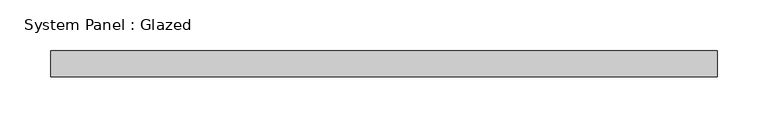
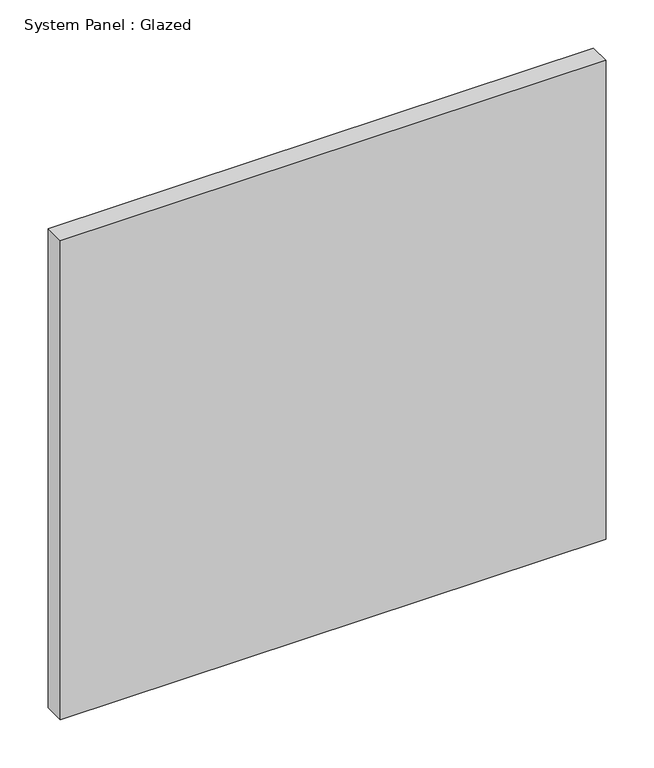
"""IFC4 building model written with IfcOpenShell, lengths in millimetres: plate geometry, System Panel : Glazed."""

from ifc_helpers import new_model, si_unit, origin, origin_with_axes, place, context, project, spatial, polyline, outline, extrude, source, transform, mapped, element, save


def system_panel_glazed_d6f2290d(model_context):
    return source(origin(), model_context, "Body", "SweptSolid", [
        extrude(outline(polyline([(327.0977679, 19.05), (-327.0977679, 19.05), (-327.0977679, 44.45), (327.0977679, 44.45), (327.0977679, 19.05)])), origin_with_axes(), (0.0, 0.0, 1.0), 606.976051),
    ])


if __name__ == "__main__":
    model = new_model("IFC4")
    model_context = context("Model", 3, world=origin())
    ifc_project = project(units=[si_unit("LENGTHUNIT", "METRE", prefix="MILLI")], contexts=[model_context])
    site = spatial("IfcSite", under=ifc_project)
    building = spatial("IfcBuilding", under=site)
    placement = place(None, origin())
    system_panel_glazed_shape = system_panel_glazed_d6f2290d(model_context)
    element("IfcPlate", 1, ObjectType="System Panel : Glazed", at=placement, inside=building, context=model_context, shape_type="MappedRepresentation", body=[
        mapped(system_panel_glazed_shape, transform((0.0, 0.0, 0.0), x_axis=(1.0, 0.0, 0.0), y_axis=(0.0, 1.0, 0.0), z_axis=(0.0, 0.0, 1.0))),
    ])
    save(model, "model.ifc")

# Revit data of these elements
# Type "System Panel : Glazed"
#   Construction Type Id = "GSP4R"
#   Analytic Construction = "1/8 in Pilkington single glazing"
#   Visual Light Transmittance = 0.9
#   Solar Heat Gain Coefficient = 0.86
#   Heat Transfer Coefficient (U) = 1.18115 BTU/(h·ft²·°F)
#   Define Thermal Properties by = 1
# Element 1 (IfcPlate, "System Panel : Glazed")
#   Materials on its faces: "Glass"
# Materials
#   "Glass": class "Glass", colour RGB 0 128 192, transparency 0.75, Description = "Soda Lime Glass", Cost = 0
